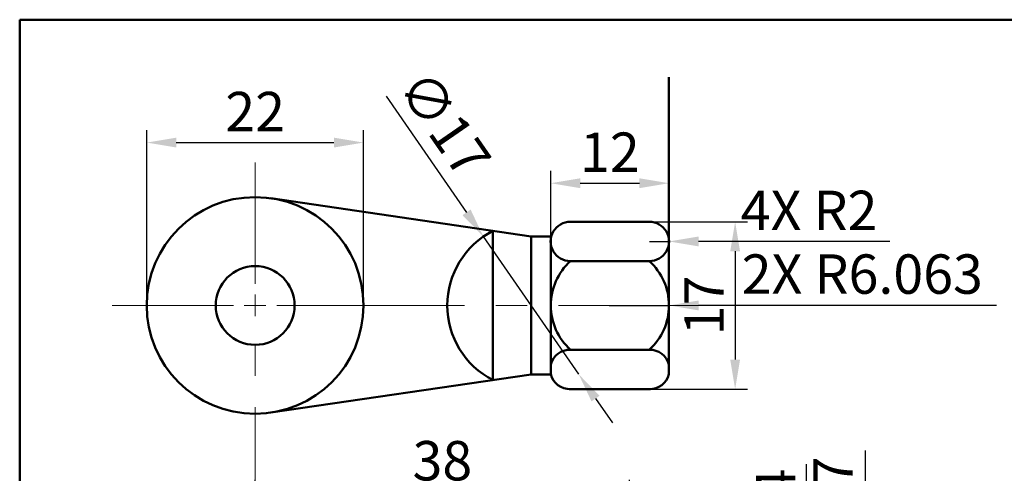
# Model space of a CAD drawing. Units: millimetres. Extents: x 139 to 291, y 28 to 164.
# Tile 4 of 5: x 140 to 240, y 118 to 164. Entities that reach past the tile are written whole.
import ezdxf

# ---------------------------------------------------------------- set-up
doc = ezdxf.new("R2010")
doc.units = ezdxf.units.MM
doc.linetypes.add('CENTER2', pattern=[28.575, 19.05, -3.175, 3.175, -3.175])
for name, color, linetype, lineweight in [('M-CNTR', 1, 'CENTER2', 18), ('M-DIMS', 2, 'Continuous', 25), ('M-OUTL', 7, 'Continuous', 50)]:
    doc.layers.add(name, color=color, linetype=linetype, lineweight=lineweight)
doc.styles.get("Standard").update_dxf_attribs({"font": 'arial.ttf'})
doc.dimstyles.new('ISO-25', dxfattribs={"dimtxt": 4, "dimasz": 3, "dimexe": 1.25, "dimexo": 0.625, "dimtad": 1, "dimdec": 0, "dimtxsty": 'Standard', "dimcen": 2.5, "dimadec": 0, "dimazin": 0, "dimtfac": 1, "dimtdec": 0, "dimtmove": 0, "dimatfit": 3, "dimfxl": 1, "dimarcsym": 0})

# ---------------------------------------------------------------- blocks, each defined once
blk = doc.blocks.new('*U1')
at = {"layer": 'M-CNTR', "color": 0, "transparency": 16777216}
for p, q in [((0, 2.2), (0, 14.5)), ((-14.5, 0), (-2.2, 0)), ((2.2, 0), (65.925, 0)), ((0, -57.955), (0, -2.2))]:
    blk.add_line(p, q, dxfattribs=at)
at = {"layer": 'M-CNTR', "color": 0, "linetype": 'Continuous', "transparency": 16777216}
for p, q in [((0, -1.1), (0, 1.1)), ((-1.1, 0), (1.1, 0))]:
    blk.add_line(p, q, dxfattribs=at)
blk = doc.blocks.new('*D4')
at = {"layer": 'Defpoints', "color": 0, "transparency": 16777216}
for p in [(201.636, 104.663), (201.636, 90.663), (219.607, 90.663)]:
    blk.add_point(p, dxfattribs=at)
at = {"layer": 'M-DIMS', "color": 0, "lineweight": -2, "transparency": 16777216}
for p, q in [((219.607, 104.663), (219.607, 119.099)), ((202.261, 104.663), (220.857, 104.663)), ((219.607, 93.663), (219.607, 101.663)), ((202.261, 90.663), (220.857, 90.663))]:
    blk.add_line(p, q, dxfattribs=at)
at = {"layer": 'M-DIMS', "color": 0, "transparency": 16777216}
for points in [[(219.107, 101.663), (220.107, 101.663), (219.607, 104.663)], [(219.107, 93.663), (220.107, 93.663), (219.607, 90.663)]]:
    blk.add_solid(points, dxfattribs=at)
at = {"layer": 'M-DIMS', "color": 0, "transparency": 16777216, "insert": (216.974, 113.381), "char_height": 4, "attachment_point": 5, "rotation": 90}
blk.add_mtext('M14', dxfattribs=at)
blk = doc.blocks.new('*D5')
at = {"layer": 'Defpoints', "color": 0, "transparency": 16777216}
for p in [(205.636, 106.163), (205.636, 89.163), (225.591, 89.163)]:
    blk.add_point(p, dxfattribs=at)
at = {"layer": 'M-DIMS', "color": 0, "lineweight": -2, "transparency": 16777216}
for p, q in [((225.591, 106.163), (225.591, 120.495)), ((206.261, 106.163), (226.841, 106.163)), ((225.591, 92.163), (225.591, 103.163)), ((206.261, 89.163), (226.841, 89.163))]:
    blk.add_line(p, q, dxfattribs=at)
at = {"layer": 'M-DIMS', "color": 0, "transparency": 16777216}
for points in [[(225.091, 103.163), (226.091, 103.163), (225.591, 106.163)], [(225.091, 92.163), (226.091, 92.163), (225.591, 89.163)]]:
    blk.add_solid(points, dxfattribs=at)
at = {"layer": 'M-DIMS', "color": 0, "transparency": 16777216, "insert": (222.811, 114.829), "char_height": 4, "attachment_point": 5, "rotation": 90}
blk.add_mtext('%%C17', dxfattribs=at)
blk = doc.blocks.new('*D6')
at = {"layer": 'Defpoints', "color": 0, "transparency": 16777216}
for p in [(163.636, 116.256), (163.636, 110.703), (201.636, 110.703)]:
    blk.add_point(p, dxfattribs=at)
at = {"layer": 'M-DIMS', "color": 0, "lineweight": -2, "transparency": 16777216}
for p, q in [((163.636, 111.328), (163.636, 117.506)), ((201.636, 111.328), (201.636, 117.506)), ((198.636, 116.256), (166.636, 116.256))]:
    blk.add_line(p, q, dxfattribs=at)
at = {"layer": 'M-DIMS', "color": 0, "transparency": 16777216}
for points in [[(166.636, 116.756), (166.636, 115.756), (163.636, 116.256)], [(198.636, 116.756), (198.636, 115.756), (201.636, 116.256)]]:
    blk.add_solid(points, dxfattribs=at)
at = {"layer": 'M-DIMS', "color": 0, "transparency": 16777216, "insert": (182.636, 118.925), "char_height": 4, "attachment_point": 5}
blk.add_mtext('38', dxfattribs=at)
blk = doc.blocks.new('*D14')
at = {"layer": 'Defpoints', "color": 0, "transparency": 16777216}
for p in [(186.798, 142.202), (196.474, 128.225)]:
    blk.add_point(p, dxfattribs=at)
at = {"layer": 'M-DIMS', "color": 0, "lineweight": -2, "transparency": 16777216}
for p, q in [((176.932, 156.452), (185.09, 144.668)), ((196.474, 128.225), (186.798, 142.202)), ((198.182, 125.758), (199.889, 123.291))]:
    blk.add_line(p, q, dxfattribs=at)
at = {"layer": 'M-DIMS', "color": 0, "transparency": 16777216}
for points in [[(185.501, 144.953), (184.679, 144.384), (186.798, 142.202)], [(198.593, 126.043), (197.771, 125.473), (196.474, 128.225)]]:
    blk.add_solid(points, dxfattribs=at)
at = {"layer": 'M-DIMS', "color": 0, "transparency": 16777216, "insert": (182.442, 153.375), "char_height": 4, "attachment_point": 5, "rotation": 304.6953}
blk.add_mtext('∅17', dxfattribs=at)
blk = doc.blocks.new('*D15')
at = {"layer": 'Defpoints', "color": 0, "transparency": 16777216}
for p in [(205.636, 147.625), (193.636, 141.501), (205.636, 141.501)]:
    blk.add_point(p, dxfattribs=at)
at = {"layer": 'M-DIMS', "color": 0, "lineweight": -2, "transparency": 16777216}
for p, q in [((193.636, 142.126), (193.636, 148.875)), ((205.636, 142.126), (205.636, 148.875)), ((196.636, 147.625), (202.636, 147.625))]:
    blk.add_line(p, q, dxfattribs=at)
at = {"layer": 'M-DIMS', "color": 0, "transparency": 16777216}
for points in [[(196.636, 148.125), (196.636, 147.125), (193.636, 147.625)], [(202.636, 148.125), (202.636, 147.125), (205.636, 147.625)]]:
    blk.add_solid(points, dxfattribs=at)
at = {"layer": 'M-DIMS', "color": 0, "transparency": 16777216, "insert": (199.636, 150.258), "char_height": 4, "attachment_point": 5}
blk.add_mtext('12', dxfattribs=at)
blk = doc.blocks.new('*D16')
at = {"layer": 'Defpoints', "color": 0, "transparency": 16777216}
for p in [(199.636, 143.713), (199.636, 126.713), (212.351, 126.713)]:
    blk.add_point(p, dxfattribs=at)
at = {"layer": 'M-DIMS', "color": 0, "lineweight": -2, "transparency": 16777216}
for p, q in [((200.261, 143.713), (213.601, 143.713)), ((212.351, 140.713), (212.351, 129.713)), ((200.261, 126.713), (213.601, 126.713))]:
    blk.add_line(p, q, dxfattribs=at)
at = {"layer": 'M-DIMS', "color": 0, "transparency": 16777216}
for points in [[(211.851, 140.713), (212.851, 140.713), (212.351, 143.713)], [(211.851, 129.713), (212.851, 129.713), (212.351, 126.713)]]:
    blk.add_solid(points, dxfattribs=at)
at = {"layer": 'M-DIMS', "color": 0, "transparency": 16777216, "insert": (209.718, 135.213), "char_height": 4, "attachment_point": 5, "rotation": 90}
blk.add_mtext('17', dxfattribs=at)
blk = doc.blocks.new('*D17')
at = {"layer": 'Defpoints', "color": 0, "transparency": 16777216}
for p in [(174.636, 151.752), (152.636, 135.213), (174.636, 135.213)]:
    blk.add_point(p, dxfattribs=at)
at = {"layer": 'M-DIMS', "color": 0, "lineweight": -2, "transparency": 16777216}
for p, q in [((152.636, 135.838), (152.636, 153.002)), ((174.636, 135.838), (174.636, 153.002)), ((155.636, 151.752), (171.636, 151.752))]:
    blk.add_line(p, q, dxfattribs=at)
at = {"layer": 'M-DIMS', "color": 0, "transparency": 16777216}
for points in [[(155.636, 152.252), (155.636, 151.252), (152.636, 151.752)], [(171.636, 152.252), (171.636, 151.252), (174.636, 151.752)]]:
    blk.add_solid(points, dxfattribs=at)
at = {"layer": 'M-DIMS', "color": 0, "transparency": 16777216, "insert": (163.636, 154.385), "char_height": 4, "attachment_point": 5}
blk.add_mtext('22', dxfattribs=at)
blk = doc.blocks.new('*D58')
at = {"layer": 'Defpoints', "color": 0, "transparency": 16777216}
for p in [(199.573, 135.213), (205.636, 135.213)]:
    blk.add_point(p, dxfattribs=at)
at = {"layer": 'M-DIMS', "color": 0, "lineweight": -2, "transparency": 16777216}
for p, q in [((199.573, 135.213), (205.636, 135.213)), ((238.875, 135.212), (208.636, 135.213))]:
    blk.add_line(p, q, dxfattribs=at)
at = {"layer": 'M-DIMS', "color": 0, "transparency": 16777216}
blk.add_solid([(208.636, 135.713), (208.636, 134.713), (205.636, 135.213)], dxfattribs=at)
at = {"layer": 'M-DIMS', "color": 0, "transparency": 16777216, "insert": (225.255, 137.881), "char_height": 4, "attachment_point": 5, "rotation": 359.99815}
blk.add_mtext('2X R6.063', dxfattribs=at)
blk = doc.blocks.new('*D59')
at = {"layer": 'Defpoints', "color": 0, "transparency": 16777216}
for p in [(203.647, 141.713), (205.647, 141.713)]:
    blk.add_point(p, dxfattribs=at)
at = {"layer": 'M-DIMS', "color": 0, "lineweight": -2, "transparency": 16777216}
for p, q in [((203.647, 141.713), (205.647, 141.713)), ((228.062, 141.711), (208.647, 141.713))]:
    blk.add_line(p, q, dxfattribs=at)
at = {"layer": 'M-DIMS', "color": 0, "transparency": 16777216}
blk.add_solid([(208.647, 142.213), (208.647, 141.213), (205.647, 141.713)], dxfattribs=at)
at = {"layer": 'M-DIMS', "color": 0, "transparency": 16777216, "insert": (219.855, 144.346), "char_height": 4, "attachment_point": 5, "rotation": 359.99439}
blk.add_mtext('4X R2', dxfattribs=at)

msp = doc.modelspace()

# ---------------------------------------------------------------- linework, layer by layer
at = {"layer": 'M-OUTL'}
for p, q in [((205.6359, 158.4068), (205.6359, 128.2253)), ((165.2366, 146.0961), (191.6359, 142.2132)), ((203.6584, 143.7132), (195.6133, 143.7132)), ((187.7679, 142.7821), (187.7679, 127.6443)), ((193.6359, 142.2132), (191.6359, 142.2132)), ((191.6359, 142.2132), (191.6359, 128.2132)), ((193.6359, 141.9255), (193.6359, 128.2253)), ((205.6359, 128.2253), (205.6359, 141.9255)), ((203.6584, 139.7132), (195.6133, 139.7132)), ((203.7549, 130.7132), (195.5168, 130.7132)), ((165.2366, 124.3303), (191.6359, 128.2132)), ((191.6359, 128.2132), (193.6389, 128.2132)), ((195.5168, 126.7132), (203.7549, 126.7132))]:
    msp.add_line(p, q, dxfattribs=at)
msp.add_lwpolyline([(139.74, 164.2339), (291.244, 164.2339), (291.244, 28.1944), (139.74, 28.1944)], close=True, dxfattribs=at)
for radius in [11, 4]:
    msp.add_circle((163.6359, 135.2132), radius, dxfattribs=at)
for centre, radius, start, end in [((195.6246, 141.7132), 2, 89.677332, 270.322668), ((203.6471, 141.7132), 2, 269.677332, 90.322668), ((191.6359, 135.2132), 8.5, 117.068734, 242.931266), ((199.6984, 135.2132), 6.0625, 132.075022, 227.924978), ((199.5734, 135.2132), 6.0625, 312.075022, 47.924978), ((195.5763, 128.7132), 2.0009, 88.295425, 165.885789), ((203.6954, 128.7132), 2.0009, 14.114211, 91.704575), ((195.5763, 128.7132), 2.0009, 194.114211, 271.70457), ((203.6954, 128.7132), 2.0009, 268.29543, 345.885789)]:
    msp.add_arc(centre, radius, start, end, dxfattribs=at)

# ---------------------------------------------------------------- block references
at = {"layer": 'M-CNTR'}
msp.add_blockref('*U1', (163.6359, 135.2132), dxfattribs=at)

# ---------------------------------------------------------------- dimensions: what is measured, and where the dimension line sits
at = {"layer": 'M-DIMS'}
dim = msp.add_diameter_dim_2p(p1=(196.4742, 128.2246), p2=(186.7975, 142.2018), dimstyle='ISO-25', override={"dimclrd": 0, "dimclre": 0, "dimclrt": 0}, dxfattribs=at)
dim.commit()
dim.dimension.update_dxf_attribs({"geometry": '*D14', "text_midpoint": (182.4422, 153.3754)})
for base, p1, p2, picture, middle in [((174.6359, 151.7521), (152.6359, 135.2132), (174.6359, 135.2132), '*D17', (163.6359, 154.3853)), ((205.6359, 147.6252), (193.6359, 141.5009), (205.6359, 141.5009), '*D15', (199.6359, 150.2584)), ((163.6359, 116.2564), (201.6359, 110.7027), (163.6359, 110.7027), '*D6', (182.6359, 118.9251))]:
    dim = msp.add_linear_dim(base=base, p1=p1, p2=p2, dimstyle='ISO-25', override={"dimclrd": 0, "dimclre": 0, "dimclrt": 0}, dxfattribs=at)
    dim.commit()
    dim.dimension.update_dxf_attribs({"geometry": picture, "text_midpoint": middle})
for center, mpoint, text, override, picture, middle in [((203.6471, 141.7132), (205.6471, 141.713), '4X <>', {"dimdec": 0, "dimlfac": 1, "dimrnd": 0, "dimzin": 0, "dimdsep": 46, "dimlunit": 2}, '*D59', (219.8549, 144.3462)), ((199.573352, 135.213196), (205.635852, 135.213), '2X <>', {"dimdec": 3, "dimlfac": 1, "dimrnd": 0, "dimzin": 0, "dimdsep": 46, "dimlunit": 2}, '*D58', (225.2554812412, 137.8810219082))]:
    dim = msp.add_radius_dim(center=center, mpoint=mpoint, text=text, dimstyle='ISO-25', override=override, dxfattribs=at)
    dim.commit()
    dim.dimension.update_dxf_attribs({"geometry": picture, "text_midpoint": middle})
dim = msp.add_linear_dim(base=(212.3514, 126.7132), p1=(199.6359, 143.7132), p2=(199.6359, 126.7132), angle=90, dimstyle='ISO-25', override={"dimclrd": 0, "dimclre": 0, "dimclrt": 0}, dxfattribs=at)
dim.commit()
dim.dimension.update_dxf_attribs({"geometry": '*D16', "text_midpoint": (209.7182, 135.2132)})
for base, p1, p2, text, picture, middle in [((225.5906, 89.1632), (205.6359, 106.1632), (205.6359, 89.1632), '%%C<>', '*D5', (225.5906, 114.8292)), ((219.6067, 90.6632), (201.6359, 104.6632), (201.6359, 90.6632), 'M<>', '*D4', (219.6067, 113.381))]:
    dim = msp.add_linear_dim(base=base, p1=p1, p2=p2, angle=90, text=text, dimstyle='ISO-25', override={"dimclrd": 0, "dimclre": 0, "dimclrt": 0}, dxfattribs=at)
    dim.commit()
    dim.dimension.update_dxf_attribs({"geometry": picture, "text_midpoint": middle, "dimtype": 160})

doc.saveas('drawing.dxf')
